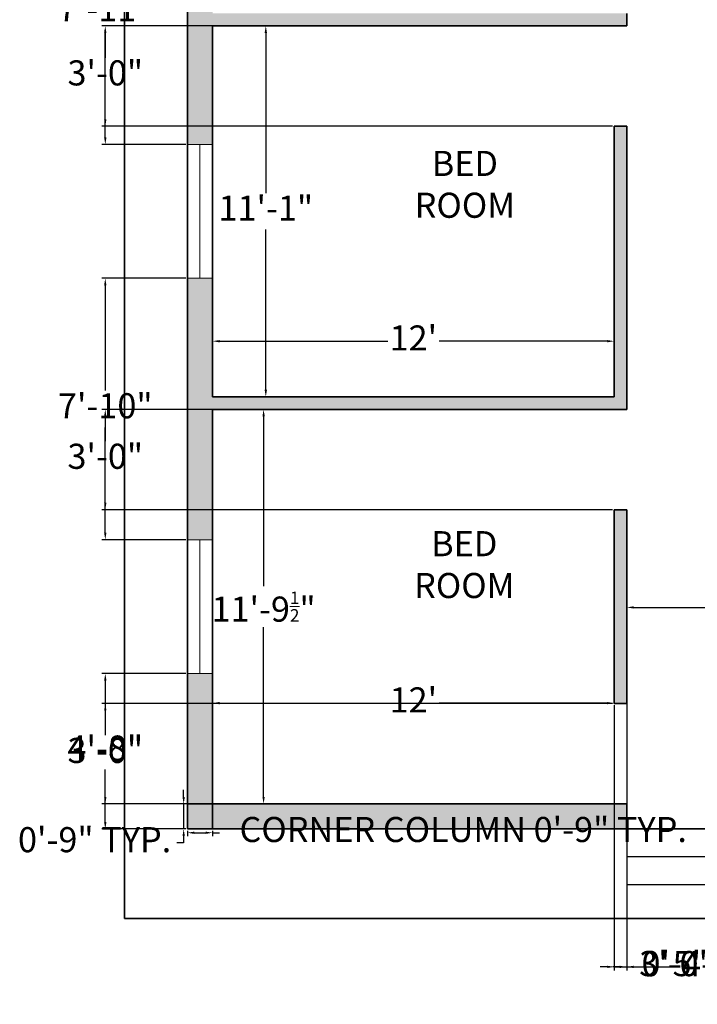
# Model space of a CAD drawing. Units: inches. Extents: x 4987 to 5457, y 8145 to 8785.
# Tile 1 of 3: x 4994 to 5237, y 8145 to 8498. Entities that reach past the tile are written whole.
import ezdxf

# ---------------------------------------------------------------- set-up
doc = ezdxf.new("R2010")
doc.units = ezdxf.units.IN
for name, color, linetype, lineweight in [('A-ANNO-DIMS', 2, 'Continuous', 18), ('A-ANNO-TTLB', 7, 'Continuous', 35), ('A-AREA-IDEN', 240, 'Continuous', 25), ('A-COLS', 7, 'Continuous', 35), ('A-COLS-PATT', 7, 'Continuous', 13), ('A-FLOR-STRS', 7, 'Continuous', 25), ('A-GLAZ', 4, 'Continuous', 18), ('A-WALL', 7, 'Continuous', 35)]:
    doc.layers.add(name, color=color, linetype=linetype, lineweight=lineweight)
doc.layers.add('A-WALL-PATT', color=67, linetype='Continuous', lineweight=13, true_color=0x727430)
doc.styles.get("Standard").update_dxf_attribs({"font": 'arial.ttf'})
doc.dimstyles.new('ISO-25', dxfattribs={"dimtxt": 9, "dimasz": 2.5, "dimexe": 1.25, "dimexo": 0.625, "dimgap": 2, "dimtad": 0, "dimtih": 1, "dimtoh": 1, "dimdec": 1, "dimlunit": 4, "dimtxsty": 'Standard', "dimcen": 2.5, "dimadec": 0, "dimazin": 0, "dimtfac": 0.5, "dimtdec": 1, "dimtmove": 0, "dimatfit": 3, "dimfxl": 1, "dimarcsym": 0})

# ---------------------------------------------------------------- blocks, each defined once
blk = doc.blocks.new('*D9')
at = {"layer": 'A-ANNO-DIMS', "color": 0, "lineweight": -2, "transparency": 16777216}
for p, q in [((5063.47, 8495.74), (5083.19, 8495.74)), ((5081.94, 8493.24), (5081.94, 8435.75)), ((5081.94, 8365.24), (5081.94, 8422.72)), ((5063.47, 8362.74), (5083.19, 8362.74))]:
    blk.add_line(p, q, dxfattribs=at)
at = {"layer": 'A-ANNO-DIMS', "color": 0, "transparency": 16777216}
for points in [[(5081.52, 8493.24), (5082.36, 8493.24), (5081.94, 8495.74)], [(5081.52, 8365.24), (5082.36, 8365.24), (5081.94, 8362.74)]]:
    blk.add_solid(points, dxfattribs=at)
at = {"layer": 'Defpoints', "color": 0, "transparency": 16777216}
for p in [(5062.84, 8495.74), (5062.84, 8362.74), (5081.94, 8362.74)]:
    blk.add_point(p, dxfattribs=at)
at = {"layer": 'A-ANNO-DIMS', "color": 0, "transparency": 16777216, "insert": (5081.94, 8429.24), "char_height": 9, "attachment_point": 5}
blk.add_mtext('11\'-1"', dxfattribs=at)
blk = doc.blocks.new('*D10')
at = {"layer": 'A-ANNO-DIMS', "color": 0, "lineweight": -2, "transparency": 16777216}
for p, q in [((5062.84, 8363.36), (5062.84, 8383.93)), ((5206.84, 8363.36), (5206.84, 8383.93)), ((5065.34, 8382.68), (5125.63, 8382.68)), ((5204.34, 8382.68), (5144.05, 8382.68))]:
    blk.add_line(p, q, dxfattribs=at)
at = {"layer": 'A-ANNO-DIMS', "color": 0, "transparency": 16777216}
for points in [[(5065.34, 8383.09), (5065.34, 8382.26), (5062.84, 8382.68)], [(5204.34, 8383.09), (5204.34, 8382.26), (5206.84, 8382.68)]]:
    blk.add_solid(points, dxfattribs=at)
at = {"layer": 'Defpoints', "color": 0, "transparency": 16777216}
for p in [(5206.84, 8382.68), (5062.84, 8362.74), (5206.84, 8362.74)]:
    blk.add_point(p, dxfattribs=at)
at = {"layer": 'A-ANNO-DIMS', "color": 0, "transparency": 16777216, "insert": (5134.84, 8382.68), "char_height": 9, "attachment_point": 5}
blk.add_mtext("12'", dxfattribs=at)
blk = doc.blocks.new('*D16')
at = {"layer": 'A-ANNO-DIMS', "color": 0, "lineweight": -2, "transparency": 16777216}
for p, q in [((5211.34, 8300.11), (5211.34, 8285.95)), ((5380.84, 8300.11), (5380.84, 8285.95)), ((5213.84, 8287.2), (5277.41, 8287.2)), ((5378.34, 8287.2), (5314.77, 8287.2))]:
    blk.add_line(p, q, dxfattribs=at)
at = {"layer": 'A-ANNO-DIMS', "color": 0, "transparency": 16777216}
for points in [[(5213.84, 8287.62), (5213.84, 8286.79), (5211.34, 8287.2)], [(5378.34, 8287.62), (5378.34, 8286.79), (5380.84, 8287.2)]]:
    blk.add_solid(points, dxfattribs=at)
at = {"layer": 'Defpoints', "color": 0, "transparency": 16777216}
for p in [(5211.34, 8300.74), (5380.84, 8300.74), (5211.34, 8287.2)]:
    blk.add_point(p, dxfattribs=at)
at = {"layer": 'A-ANNO-DIMS', "color": 0, "transparency": 16777216, "insert": (5296.09, 8287.2), "char_height": 9, "attachment_point": 5}
blk.add_mtext('14\'-1{\\H0.5x;\\S1/2;}"', dxfattribs=at)
blk = doc.blocks.new('*D17')
at = {"layer": 'A-ANNO-DIMS', "color": 0, "lineweight": -2, "transparency": 16777216}
for p, q in [((5063.47, 8358.24), (5082.39, 8358.24)), ((5081.14, 8355.74), (5081.14, 8294.83)), ((5081.14, 8219.24), (5081.14, 8280.14)), ((5063.47, 8216.74), (5082.39, 8216.74))]:
    blk.add_line(p, q, dxfattribs=at)
at = {"layer": 'A-ANNO-DIMS', "color": 0, "transparency": 16777216}
for points in [[(5080.73, 8355.74), (5081.56, 8355.74), (5081.14, 8358.24)], [(5080.73, 8219.24), (5081.56, 8219.24), (5081.14, 8216.74)]]:
    blk.add_solid(points, dxfattribs=at)
at = {"layer": 'Defpoints', "color": 0, "transparency": 16777216}
for p in [(5062.84, 8358.24), (5081.14, 8358.24), (5062.84, 8216.74)]:
    blk.add_point(p, dxfattribs=at)
at = {"layer": 'A-ANNO-DIMS', "color": 0, "transparency": 16777216, "insert": (5081.14, 8287.49), "char_height": 9, "attachment_point": 5}
blk.add_mtext('11\'-9{\\H0.5x;\\S1/2;}"', dxfattribs=at)
blk = doc.blocks.new('*D18')
at = {"layer": 'A-ANNO-DIMS', "color": 0, "lineweight": -2, "transparency": 16777216}
for p, q in [((5062.84, 8253.36), (5062.84, 8254.12)), ((5065.34, 8252.87), (5125.63, 8252.87)), ((5204.34, 8252.87), (5144.05, 8252.87)), ((5206.84, 8253.36), (5206.84, 8254.12))]:
    blk.add_line(p, q, dxfattribs=at)
at = {"layer": 'A-ANNO-DIMS', "color": 0, "transparency": 16777216}
for points in [[(5065.34, 8253.29), (5065.34, 8252.46), (5062.84, 8252.87)], [(5204.34, 8253.29), (5204.34, 8252.46), (5206.84, 8252.87)]]:
    blk.add_solid(points, dxfattribs=at)
at = {"layer": 'Defpoints', "color": 0, "transparency": 16777216}
for p in [(5062.84, 8252.87), (5062.84, 8252.74), (5206.84, 8252.74)]:
    blk.add_point(p, dxfattribs=at)
at = {"layer": 'A-ANNO-DIMS', "color": 0, "transparency": 16777216, "insert": (5134.84, 8252.87), "char_height": 9, "attachment_point": 5}
blk.add_mtext("12'", dxfattribs=at)
blk = doc.blocks.new('WIN-48IN')
for p, q in [((0, 0), (0, 9)), ((48, 0), (48, 9)), ((0, 4.5), (48, 4.5))]:
    blk.add_line(p, q)
blk = doc.blocks.new('COL-CORNER-9IN')
for q in [(0, 0), (9, 9)]:
    blk.add_line((0, 9), q)
blk = doc.blocks.new('*D28')
at = {"layer": 'A-ANNO-DIMS', "color": 0, "lineweight": -2, "transparency": 16777216}
for p, q in [((5053.84, 8207.11), (5053.84, 8205.14)), ((5062.84, 8207.11), (5062.84, 8205.14)), ((5056.34, 8206.39), (5060.34, 8206.39)), ((5062.84, 8206.39), (5065.34, 8206.39))]:
    blk.add_line(p, q, dxfattribs=at)
at = {"layer": 'A-ANNO-DIMS', "color": 0, "transparency": 16777216}
for points in [[(5056.34, 8206.8), (5056.34, 8205.97), (5053.84, 8206.39)], [(5060.34, 8206.8), (5060.34, 8205.97), (5062.84, 8206.39)]]:
    blk.add_solid(points, dxfattribs=at)
at = {"layer": 'Defpoints', "color": 0, "transparency": 16777216}
for p in [(5053.84, 8207.74), (5062.84, 8207.74), (5062.84, 8206.39)]:
    blk.add_point(p, dxfattribs=at)
at = {"layer": 'A-ANNO-DIMS', "color": 0, "transparency": 16777216, "insert": (5152.7, 8206.39), "char_height": 9, "attachment_point": 5}
blk.add_mtext('CORNER COLUMN 0\'-9" TYP.', dxfattribs=at)
blk = doc.blocks.new('*D29')
at = {"layer": 'A-ANNO-DIMS', "color": 0, "lineweight": -2, "transparency": 16777216}
for p, q in [((5052.49, 8219.24), (5052.49, 8221.74)), ((5053.22, 8216.74), (5051.24, 8216.74)), ((5052.49, 8216.74), (5052.49, 8207.74)), ((5053.22, 8207.74), (5051.24, 8207.74)), ((5052.49, 8205.24), (5052.49, 8202.74)), ((5052.49, 8202.74), (5049.99, 8202.74))]:
    blk.add_line(p, q, dxfattribs=at)
at = {"layer": 'A-ANNO-DIMS', "color": 0, "transparency": 16777216}
for points in [[(5052.07, 8219.24), (5052.91, 8219.24), (5052.49, 8216.74)], [(5052.07, 8205.24), (5052.91, 8205.24), (5052.49, 8207.74)]]:
    blk.add_solid(points, dxfattribs=at)
at = {"layer": 'Defpoints', "color": 0, "transparency": 16777216}
for p in [(5053.84, 8216.74), (5052.49, 8207.74), (5053.84, 8207.74)]:
    blk.add_point(p, dxfattribs=at)
at = {"layer": 'A-ANNO-DIMS', "color": 0, "transparency": 16777216, "insert": (5020.56, 8202.74), "char_height": 9, "attachment_point": 5}
blk.add_mtext('0\'-9" TYP.', dxfattribs=at)
blk = doc.blocks.new('*D30')
at = {"layer": 'A-ANNO-DIMS', "color": 0, "lineweight": -2, "transparency": 16777216}
for p, q in [((5053.22, 8263.49), (5023.14, 8263.49)), ((5024.39, 8260.99), (5024.39, 8242.21)), ((5024.39, 8210.24), (5024.39, 8229.02)), ((5053.22, 8207.74), (5023.14, 8207.74))]:
    blk.add_line(p, q, dxfattribs=at)
at = {"layer": 'A-ANNO-DIMS', "color": 0, "transparency": 16777216}
for points in [[(5023.97, 8260.99), (5024.81, 8260.99), (5024.39, 8263.49)], [(5023.97, 8210.24), (5024.81, 8210.24), (5024.39, 8207.74)]]:
    blk.add_solid(points, dxfattribs=at)
at = {"layer": 'Defpoints', "color": 0, "transparency": 16777216}
for p in [(5024.39, 8263.49), (5053.84, 8263.49), (5053.84, 8207.74)]:
    blk.add_point(p, dxfattribs=at)
at = {"layer": 'A-ANNO-DIMS', "color": 0, "transparency": 16777216, "insert": (5024.39, 8235.61), "char_height": 9, "attachment_point": 5}
blk.add_mtext('4\'-8"', dxfattribs=at)
blk = doc.blocks.new('*D31')
at = {"layer": 'A-ANNO-DIMS', "color": 0, "lineweight": -2, "transparency": 16777216}
for p, q in [((5053.22, 8405.24), (5023.14, 8405.24)), ((5024.39, 8402.74), (5024.39, 8364.96)), ((5024.39, 8313.99), (5024.39, 8351.77)), ((5053.22, 8311.49), (5023.14, 8311.49))]:
    blk.add_line(p, q, dxfattribs=at)
at = {"layer": 'A-ANNO-DIMS', "color": 0, "transparency": 16777216}
for points in [[(5023.97, 8402.74), (5024.81, 8402.74), (5024.39, 8405.24)], [(5023.97, 8313.99), (5024.81, 8313.99), (5024.39, 8311.49)]]:
    blk.add_solid(points, dxfattribs=at)
at = {"layer": 'Defpoints', "color": 0, "transparency": 16777216}
for p in [(5024.39, 8405.24), (5053.84, 8405.24), (5053.84, 8311.49)]:
    blk.add_point(p, dxfattribs=at)
at = {"layer": 'A-ANNO-DIMS', "color": 0, "transparency": 16777216, "insert": (5024.39, 8358.36), "char_height": 9, "attachment_point": 5}
blk.add_mtext('7\'-10"', dxfattribs=at)
blk = doc.blocks.new('*D32')
at = {"layer": 'A-ANNO-DIMS', "color": 0, "lineweight": -2, "transparency": 16777216}
for p, q in [((5053.22, 8548.24), (5023.14, 8548.24)), ((5024.39, 8545.74), (5024.39, 8507.25)), ((5024.39, 8455.74), (5024.39, 8494.22)), ((5053.22, 8453.24), (5023.14, 8453.24))]:
    blk.add_line(p, q, dxfattribs=at)
at = {"layer": 'A-ANNO-DIMS', "color": 0, "transparency": 16777216}
for points in [[(5023.97, 8545.74), (5024.81, 8545.74), (5024.39, 8548.24)], [(5023.97, 8455.74), (5024.81, 8455.74), (5024.39, 8453.24)]]:
    blk.add_solid(points, dxfattribs=at)
at = {"layer": 'Defpoints', "color": 0, "transparency": 16777216}
for p in [(5024.39, 8548.24), (5053.84, 8548.24), (5053.84, 8453.24)]:
    blk.add_point(p, dxfattribs=at)
at = {"layer": 'A-ANNO-DIMS', "color": 0, "transparency": 16777216, "insert": (5024.39, 8500.74), "char_height": 9, "attachment_point": 5}
blk.add_mtext('7\'-11"', dxfattribs=at)
blk = doc.blocks.new('*D37')
at = {"layer": 'A-ANNO-DIMS', "color": 0, "lineweight": -2, "transparency": 16777216}
for p, q in [((5211.34, 8187.11), (5211.34, 8157.04)), ((5271.34, 8187.11), (5271.34, 8157.04)), ((5213.84, 8158.29), (5227.38, 8158.29)), ((5268.84, 8158.29), (5255.3, 8158.29))]:
    blk.add_line(p, q, dxfattribs=at)
at = {"layer": 'A-ANNO-DIMS', "color": 0, "transparency": 16777216}
for points in [[(5213.84, 8158.7), (5213.84, 8157.87), (5211.34, 8158.29)], [(5268.84, 8158.7), (5268.84, 8157.87), (5271.34, 8158.29)]]:
    blk.add_solid(points, dxfattribs=at)
at = {"layer": 'Defpoints', "color": 0, "transparency": 16777216}
for p in [(5211.34, 8187.74), (5271.34, 8187.74), (5271.34, 8158.29)]:
    blk.add_point(p, dxfattribs=at)
at = {"layer": 'A-ANNO-DIMS', "color": 0, "transparency": 16777216, "insert": (5241.34, 8158.29), "char_height": 9, "attachment_point": 5}
blk.add_mtext('5\'-0"', dxfattribs=at)
blk = doc.blocks.new('*D46')
at = {"layer": 'A-ANNO-DIMS', "color": 0, "lineweight": -2, "transparency": 16777216}
for p, q in [((5206.22, 8495.74), (5023.14, 8495.74)), ((5024.39, 8493.24), (5024.39, 8484.33)), ((5024.39, 8462.24), (5024.39, 8471.14)), ((5206.22, 8459.74), (5023.14, 8459.74))]:
    blk.add_line(p, q, dxfattribs=at)
at = {"layer": 'A-ANNO-DIMS', "color": 0, "transparency": 16777216}
for points in [[(5023.97, 8493.24), (5024.81, 8493.24), (5024.39, 8495.74)], [(5023.97, 8462.24), (5024.81, 8462.24), (5024.39, 8459.74)]]:
    blk.add_solid(points, dxfattribs=at)
at = {"layer": 'Defpoints', "color": 0, "transparency": 16777216}
for p in [(5024.39, 8495.74), (5206.84, 8495.74), (5206.84, 8459.74)]:
    blk.add_point(p, dxfattribs=at)
at = {"layer": 'A-ANNO-DIMS', "color": 0, "transparency": 16777216, "insert": (5024.39, 8477.74), "char_height": 9, "attachment_point": 5}
blk.add_mtext('3\'-0"', dxfattribs=at)
blk = doc.blocks.new('*D47')
at = {"layer": 'A-ANNO-DIMS', "color": 0, "lineweight": -2, "transparency": 16777216}
for p, q in [((5206.22, 8358.24), (5023.14, 8358.24)), ((5024.39, 8355.74), (5024.39, 8346.83)), ((5024.39, 8324.74), (5024.39, 8333.64)), ((5206.22, 8322.24), (5023.14, 8322.24))]:
    blk.add_line(p, q, dxfattribs=at)
at = {"layer": 'A-ANNO-DIMS', "color": 0, "transparency": 16777216}
for points in [[(5023.97, 8355.74), (5024.81, 8355.74), (5024.39, 8358.24)], [(5023.97, 8324.74), (5024.81, 8324.74), (5024.39, 8322.24)]]:
    blk.add_solid(points, dxfattribs=at)
at = {"layer": 'Defpoints', "color": 0, "transparency": 16777216}
for p in [(5024.39, 8358.24), (5206.84, 8358.24), (5206.84, 8322.24)]:
    blk.add_point(p, dxfattribs=at)
at = {"layer": 'A-ANNO-DIMS', "color": 0, "transparency": 16777216, "insert": (5024.39, 8340.24), "char_height": 9, "attachment_point": 5}
blk.add_mtext('3\'-0"', dxfattribs=at)
blk = doc.blocks.new('*D49')
at = {"layer": 'A-ANNO-DIMS', "color": 0, "lineweight": -2, "transparency": 16777216}
for p, q in [((5211.34, 8300.11), (5211.34, 8157.04)), ((5247.34, 8300.11), (5247.34, 8157.04)), ((5208.84, 8158.29), (5206.34, 8158.29)), ((5211.34, 8158.29), (5215.38, 8158.29)), ((5247.34, 8158.29), (5243.3, 8158.29)), ((5249.84, 8158.29), (5252.34, 8158.29))]:
    blk.add_line(p, q, dxfattribs=at)
at = {"layer": 'A-ANNO-DIMS', "color": 0, "transparency": 16777216}
for points in [[(5208.84, 8158.7), (5208.84, 8157.87), (5211.34, 8158.29)], [(5249.84, 8158.7), (5249.84, 8157.87), (5247.34, 8158.29)]]:
    blk.add_solid(points, dxfattribs=at)
at = {"layer": 'Defpoints', "color": 0, "transparency": 16777216}
for p in [(5211.34, 8300.74), (5247.34, 8300.74), (5247.34, 8158.29)]:
    blk.add_point(p, dxfattribs=at)
at = {"layer": 'A-ANNO-DIMS', "color": 0, "transparency": 16777216, "insert": (5229.34, 8158.29), "char_height": 9, "attachment_point": 5}
blk.add_mtext('3\'-0"', dxfattribs=at)
blk = doc.blocks.new('*D51')
at = {"layer": 'A-ANNO-DIMS', "color": 0, "lineweight": -2, "transparency": 16777216}
for p, q in [((5206.22, 8252.74), (5023.14, 8252.74)), ((5024.39, 8250.24), (5024.39, 8241.33)), ((5024.39, 8219.24), (5024.39, 8228.14)), ((5206.22, 8216.74), (5023.14, 8216.74))]:
    blk.add_line(p, q, dxfattribs=at)
at = {"layer": 'A-ANNO-DIMS', "color": 0, "transparency": 16777216}
for points in [[(5023.97, 8250.24), (5024.81, 8250.24), (5024.39, 8252.74)], [(5023.97, 8219.24), (5024.81, 8219.24), (5024.39, 8216.74)]]:
    blk.add_solid(points, dxfattribs=at)
at = {"layer": 'Defpoints', "color": 0, "transparency": 16777216}
for p in [(5024.39, 8252.74), (5206.84, 8252.74), (5206.84, 8216.74)]:
    blk.add_point(p, dxfattribs=at)
at = {"layer": 'A-ANNO-DIMS', "color": 0, "transparency": 16777216, "insert": (5024.39, 8234.74), "char_height": 9, "attachment_point": 5}
blk.add_mtext('3\'-0"', dxfattribs=at)
blk = doc.blocks.new('*D52')
at = {"layer": 'A-ANNO-DIMS', "color": 0, "lineweight": -2, "transparency": 16777216}
for p, q in [((5206.84, 8252.11), (5206.84, 8157.04)), ((5211.34, 8252.11), (5211.34, 8157.04)), ((5204.34, 8158.29), (5201.84, 8158.29)), ((5206.84, 8158.29), (5211.34, 8158.29)), ((5213.84, 8158.29), (5216.34, 8158.29))]:
    blk.add_line(p, q, dxfattribs=at)
at = {"layer": 'A-ANNO-DIMS', "color": 0, "transparency": 16777216}
for points in [[(5204.34, 8158.7), (5204.34, 8157.87), (5206.84, 8158.29)], [(5213.84, 8158.7), (5213.84, 8157.87), (5211.34, 8158.29)]]:
    blk.add_solid(points, dxfattribs=at)
at = {"layer": 'Defpoints', "color": 0, "transparency": 16777216}
for p in [(5206.84, 8252.74), (5211.34, 8252.74), (5211.34, 8158.29)]:
    blk.add_point(p, dxfattribs=at)
at = {"layer": 'A-ANNO-DIMS', "color": 0, "transparency": 16777216, "insert": (5240.79, 8158.29), "char_height": 9, "attachment_point": 5}
blk.add_mtext('0\'-4 1/2"', dxfattribs=at)

msp = doc.modelspace()

# ---------------------------------------------------------------- hatches: boundary and pattern name
at = {"layer": 'A-COLS-PATT'}
h = msp.add_hatch(color=256, dxfattribs=at)
h.dxf.hatch_style = 1
h.paths.add_polyline_path([(5062.84, 8735.74), (5053.84, 8735.74), (5053.84, 8726.74), (5062.84, 8726.74)])
h.paths.add_polyline_path([(5389.84, 8735.74), (5380.84, 8735.74), (5380.84, 8726.74), (5389.84, 8726.74)])
h.paths.add_polyline_path([(5389.84, 8216.74), (5380.84, 8216.74), (5380.84, 8207.74), (5389.84, 8207.74)])
h.paths.add_polyline_path([(5062.84, 8216.74), (5053.84, 8216.74), (5053.84, 8207.74), (5062.84, 8207.74)])
at = {"layer": 'A-WALL-PATT'}
h = msp.add_hatch(color=256, dxfattribs=at)
h.dxf.hatch_style = 1
h.paths.add_polyline_path([(5220.34, 8735.74), (5062.84, 8735.74), (5062.84, 8726.74), (5111.84, 8726.74), (5220.34, 8726.74)])
h.paths.add_polyline_path([(5062.84, 8548.24), (5053.84, 8548.24), (5053.84, 8453.24), (5062.84, 8453.24), (5062.84, 8495.74), (5206.84, 8495.74), (5211.34, 8495.74), (5211.34, 8500.24), (5206.84, 8500.24), (5062.84, 8500.24)])
h.paths.add_polyline_path([(5211.34, 8362.74), (5211.34, 8412.74), (5211.34, 8417.24), (5211.34, 8459.74), (5206.84, 8459.74), (5206.84, 8417.24), (5206.84, 8412.74), (5206.84, 8362.74), (5062.84, 8362.74), (5062.84, 8405.24), (5053.84, 8405.24), (5053.84, 8311.49), (5062.84, 8311.49), (5062.84, 8358.24), (5206.84, 8358.24), (5211.34, 8358.24)])
h.paths.add_polyline_path([(5062.84, 8263.49), (5053.84, 8263.49), (5053.84, 8216.74), (5062.84, 8216.74)])
h.paths.add_polyline_path([(5211.34, 8216.74), (5206.84, 8216.74), (5062.84, 8216.74), (5062.84, 8207.74), (5211.34, 8207.74)])
h.paths.add_polyline_path([(5380.84, 8216.74), (5271.34, 8216.74), (5271.34, 8207.74), (5380.84, 8207.74)])
h.paths.add_polyline_path([(5389.84, 8314.24), (5380.84, 8314.24), (5380.84, 8305.24), (5332.84, 8305.24), (5332.84, 8311.24), (5328.34, 8311.24), (5328.34, 8305.24), (5247.34, 8305.24), (5247.34, 8300.74), (5380.84, 8300.74), (5380.84, 8216.74), (5389.84, 8216.74)])
h.paths.add_polyline_path([(5389.84, 8370.24), (5380.84, 8370.24), (5380.84, 8351.74), (5328.34, 8351.74), (5320.84, 8351.74), (5320.84, 8347.24), (5328.34, 8347.24), (5332.84, 8347.24), (5380.84, 8347.24), (5380.84, 8338.24), (5389.84, 8338.24)])
h.paths.add_polyline_path([(5389.84, 8494.74), (5380.84, 8494.74), (5380.84, 8417.24), (5280.34, 8417.24), (5280.34, 8412.74), (5280.34, 8351.74), (5280.34, 8347.24), (5284.84, 8347.24), (5284.84, 8351.74), (5284.84, 8412.74), (5328.34, 8412.74), (5380.84, 8412.74), (5380.84, 8394.24), (5389.84, 8394.24)])
h.paths.add_polyline_path([(5389.84, 8726.74), (5380.84, 8726.74), (5380.84, 8624.74), (5272.84, 8624.74), (5268.34, 8624.74), (5268.34, 8620.24), (5380.84, 8620.24), (5380.84, 8542.74), (5389.84, 8542.74)])
h.paths.add_polyline_path([(5062.84, 8726.74), (5053.84, 8726.74), (5053.84, 8596.24), (5062.84, 8596.24), (5062.84, 8644.24), (5062.84, 8648.74)])
h.paths.add_polyline_path([(5302.84, 8735.74), (5268.34, 8735.74), (5268.34, 8726.74), (5268.34, 8660.74), (5272.84, 8660.74), (5272.84, 8726.74), (5302.84, 8726.74)])
h.paths.add_polyline_path([(5380.84, 8735.74), (5350.84, 8735.74), (5350.84, 8726.74), (5380.84, 8726.74)])
h.paths.add_polyline_path([(5211.34, 8648.74), (5206.84, 8648.74), (5098.84, 8648.74), (5098.84, 8644.24), (5206.84, 8644.24), (5206.84, 8624.74), (5206.84, 8536.24), (5211.34, 8536.24), (5211.34, 8620.24), (5211.34, 8624.74)])
h.paths.add_polyline_path([(5211.34, 8305.24), (5211.34, 8322.24), (5206.84, 8322.24), (5206.84, 8305.24), (5206.84, 8300.74), (5206.84, 8252.74), (5211.34, 8252.74), (5211.34, 8300.74)])

# ---------------------------------------------------------------- linework, layer by layer
at = {"layer": 'A-ANNO-TTLB'}
msp.add_lwpolyline([(5031.32, 8785.05), (5433.7, 8785.05), (5433.7, 8175.66), (5031.32, 8175.66)], close=True, dxfattribs=at)
at = {"layer": 'A-FLOR-STRS'}
for p, q in [((5211.34, 8207.74), (5211.34, 8187.74)), ((5271.34, 8197.74), (5211.34, 8197.74)), ((5271.34, 8187.74), (5211.34, 8187.74))]:
    msp.add_line(p, q, dxfattribs=at)
at = {"layer": 'A-WALL'}
for p, q in [((5053.84, 8207.74), (5053.84, 8735.74)), ((5211.34, 8500.24), (5211.34, 8495.74)), ((5062.84, 8362.74), (5062.84, 8495.74)), ((5206.84, 8495.74), (5062.84, 8495.74)), ((5206.84, 8495.74), (5211.34, 8495.74)), ((5206.84, 8459.74), (5206.84, 8417.24)), ((5206.84, 8459.74), (5211.34, 8459.74)), ((5211.34, 8459.74), (5211.34, 8417.24)), ((5206.84, 8417.24), (5206.84, 8412.74)), ((5211.34, 8417.24), (5211.34, 8412.74)), ((5206.84, 8412.74), (5206.84, 8362.74)), ((5211.34, 8412.74), (5211.34, 8362.74)), ((5206.84, 8362.74), (5062.84, 8362.74)), ((5211.34, 8358.24), (5211.34, 8362.74)), ((5062.84, 8216.74), (5062.84, 8358.24)), ((5206.84, 8358.24), (5062.84, 8358.24)), ((5206.84, 8358.24), (5211.34, 8358.24)), ((5206.84, 8322.24), (5206.84, 8305.24)), ((5206.84, 8322.24), (5211.34, 8322.24)), ((5211.34, 8305.24), (5211.34, 8322.24)), ((5206.84, 8300.74), (5206.84, 8305.24)), ((5211.34, 8305.24), (5211.34, 8300.74)), ((5206.84, 8300.74), (5206.84, 8252.74)), ((5211.34, 8300.74), (5211.34, 8252.74)), ((5206.84, 8252.74), (5211.34, 8252.74)), ((5206.84, 8216.74), (5062.84, 8216.74)), ((5206.84, 8216.74), (5211.34, 8216.74)), ((5211.34, 8216.74), (5211.34, 8207.74)), ((5389.84, 8207.74), (5053.84, 8207.74))]:
    msp.add_line(p, q, dxfattribs=at)

# ---------------------------------------------------------------- block references
at = {"layer": 'A-COLS', "rotation": 270}
msp.add_blockref('COL-CORNER-9IN', (5053.84, 8216.74), dxfattribs=at)
at = {"layer": 'A-GLAZ'}
for p, rotation in [((5062.84, 8405.23), 89.9999999999979), ((5062.84, 8263.48), 89.99999999999162)]:
    msp.add_blockref('WIN-48IN', p, dxfattribs=dict(at, rotation=rotation))

# ---------------------------------------------------------------- texts
at = {"layer": 'A-AREA-IDEN', "char_height": 9, "attachment_point": 1}
for width, insert in [(76.4162, (5115.09, 8450.94)), (88.6797, (5108.75, 8314.56))]:
    msp.add_mtext_dynamic_manual_height_columns('\\pxqc;{\\fArial|b1|i0|c0|p34;BED\\PROOM}', width=width, gutter_width=12.5, heights=[0], dxfattribs=dict(at, insert=insert))

# ---------------------------------------------------------------- dimensions: what is measured, and where the dimension line sits
at = {"layer": 'A-ANNO-DIMS'}
for base, p1, p2, override, picture, middle in [((5024.39, 8548.24), (5053.84, 8453.24), (5053.84, 8548.24), {"dimdec": 1, "dimlfac": 1, "dimrnd": 0, "dimzin": 1, "dimdsep": 46, "dimlunit": 4, "dimfrac": 2}, '*D32', (5024.39, 8500.74)), ((5024.39, 8495.74), (5206.84, 8459.74), (5206.84, 8495.74), {"dimdec": 1, "dimlfac": 1, "dimrnd": 0, "dimzin": 1, "dimdsep": 46, "dimlunit": 4, "dimfrac": 2}, '*D46', (5024.39, 8477.74)), ((5081.94, 8362.74), (5062.84, 8495.74), (5062.84, 8362.74), {"dimclrd": 0, "dimclre": 0, "dimclrt": 0}, '*D9', (5081.94, 8429.24)), ((5024.390439, 8405.235338), (5053.840439, 8311.485338), (5053.840439, 8405.235338), {"dimdec": 1, "dimlfac": 1, "dimrnd": 0, "dimzin": 1, "dimdsep": 46, "dimlunit": 4, "dimfrac": 2}, '*D31', (5024.390439, 8358.360338)), ((5024.39, 8358.24), (5206.84, 8322.24), (5206.84, 8358.24), {"dimdec": 1, "dimlfac": 1, "dimrnd": 0, "dimzin": 1, "dimdsep": 46, "dimlunit": 4, "dimfrac": 2}, '*D47', (5024.39, 8340.24)), ((5081.14, 8358.24), (5062.84, 8216.74), (5062.84, 8358.24), {"dimclrd": 0, "dimclre": 0, "dimclrt": 0}, '*D17', (5081.14, 8287.49)), ((5024.390439, 8263.485338), (5053.840439, 8207.735338), (5053.840439, 8263.485338), {"dimdec": 1, "dimlfac": 1, "dimrnd": 0, "dimzin": 1, "dimdsep": 46, "dimlunit": 4, "dimfrac": 2}, '*D30', (5024.390439, 8235.610338)), ((5024.39, 8252.74), (5206.84, 8216.74), (5206.84, 8252.74), {"dimdec": 1, "dimlfac": 1, "dimrnd": 0, "dimzin": 1, "dimdsep": 46, "dimlunit": 4, "dimfrac": 2}, '*D51', (5024.39, 8234.74))]:
    dim = msp.add_linear_dim(base=base, p1=p1, p2=p2, angle=90, dimstyle='ISO-25', override=override, dxfattribs=at)
    dim.commit()
    dim.dimension.update_dxf_attribs({"geometry": picture, "text_midpoint": middle})
for base, p1, p2, override, picture, middle in [((5206.84, 8382.68), (5062.84, 8362.74), (5206.84, 8362.74), {"dimclrd": 0, "dimclre": 0, "dimclrt": 0}, '*D10', (5134.84, 8382.68)), ((5247.34, 8158.29), (5211.34, 8300.74), (5247.34, 8300.74), {"dimdec": 1, "dimlfac": 1, "dimrnd": 0, "dimzin": 1, "dimdsep": 46, "dimlunit": 4, "dimfrac": 2}, '*D49', (5229.34, 8158.29)), ((5211.34, 8287.2), (5380.84, 8300.74), (5211.34, 8300.74), {"dimclrd": 0, "dimclre": 0, "dimclrt": 0}, '*D16', (5296.09, 8287.2)), ((5062.84, 8252.87), (5206.84, 8252.74), (5062.84, 8252.74), {"dimclrd": 0, "dimclre": 0, "dimclrt": 0}, '*D18', (5134.84, 8252.87)), ((5211.34, 8158.29), (5206.84, 8252.74), (5211.34, 8252.74), {"dimdec": 1, "dimlfac": 1, "dimrnd": 0, "dimzin": 1, "dimdsep": 46, "dimlunit": 4, "dimfrac": 2}, '*D52', (5240.79, 8158.29)), ((5271.34, 8158.29), (5211.34, 8187.74), (5271.34, 8187.74), {"dimdec": 1, "dimlfac": 1, "dimrnd": 0, "dimzin": 1, "dimdsep": 46, "dimlunit": 4, "dimfrac": 2}, '*D37', (5241.34, 8158.29))]:
    dim = msp.add_linear_dim(base=base, p1=p1, p2=p2, dimstyle='ISO-25', override=override, dxfattribs=at)
    dim.commit()
    dim.dimension.update_dxf_attribs({"geometry": picture, "text_midpoint": middle})
dim = msp.add_linear_dim(base=(5062.84, 8206.39), p1=(5053.84, 8207.74), p2=(5062.84, 8207.74), text='CORNER COLUMN <> TYP.', dimstyle='ISO-25', override={"dimdec": 1, "dimlfac": 1, "dimrnd": 0, "dimzin": 1, "dimdsep": 46, "dimlunit": 4, "dimfrac": 2}, dxfattribs=at)
dim.commit()
dim.dimension.update_dxf_attribs({"geometry": '*D28', "text_midpoint": (5152.7, 8206.39)})
dim = msp.add_linear_dim(base=(5052.49, 8207.74), p1=(5053.84, 8216.74), p2=(5053.84, 8207.74), angle=270, text='<> TYP.', dimstyle='ISO-25', override={"dimdec": 1, "dimlfac": 1, "dimrnd": 0, "dimzin": 1, "dimdsep": 46, "dimlunit": 4, "dimfrac": 2}, dxfattribs=at)
dim.commit()
dim.dimension.update_dxf_attribs({"geometry": '*D29', "text_midpoint": (5020.56, 8202.74)})

doc.saveas('drawing.dxf')
